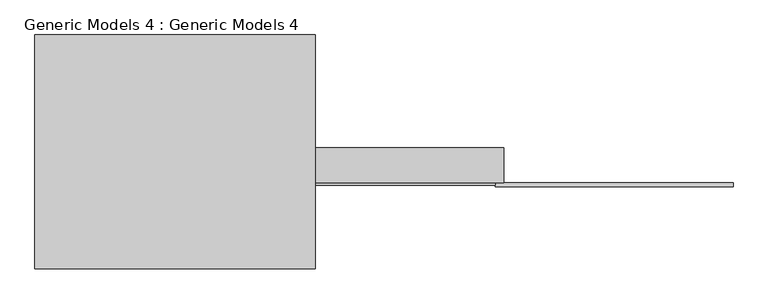
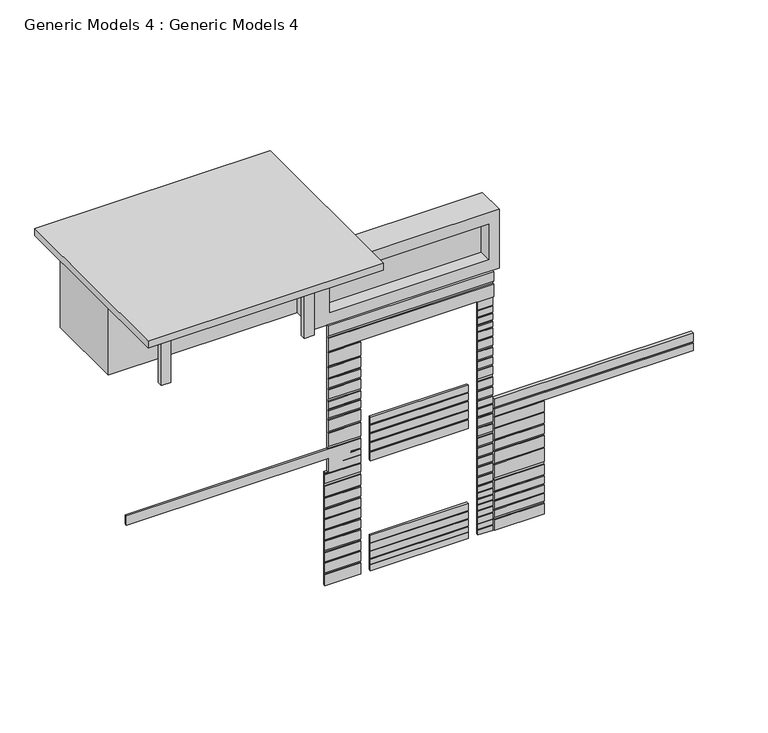
"""IFC4 building model written with IfcOpenShell, lengths in millimetres: proxy geometry, Generic Models 4 : Generic Models 4."""

from ifc_helpers import new_model, si_unit, frame, origin, place, context, project, spatial, polyline, outline, extrude, faceted_brep, source, transform, mapped, element, save


def generic_models_4_generic_models_4_71b53b29(model_context):
    return source(origin(), model_context, "Body", "SolidModel", [
        extrude(outline(polyline([(-14860.146149, 871.6720769), (-14860.146149, 0.0), (-14910.946149, 0.0), (-14910.946149, 143.2262452), (-14885.546149, 143.2262452), (-14885.546149, 160.2144956), (-14910.946149, 160.2144956), (-14910.946149, 282.4741118), (-14885.546149, 282.4741118), (-14885.546149, 303.6396643), (-14910.946149, 303.6396643), (-14910.946149, 472.2042083), (-14885.546149, 472.2042083), (-14885.546149, 489.55907), (-14910.946149, 489.55907), (-14910.946149, 670.6560858), (-14885.546149, 670.6560858), (-14885.546149, 693.359854), (-14910.946149, 693.359854), (-14910.946149, 871.6720769), (-14860.146149, 871.6720769)])), frame((-13085.9127168, 0.0, 0.0), z_axis=(1.0, 0.0, 0.0), x_axis=(0.0, 1.0, 0.0)), (0.0, 0.0, 1.0), 2286.0),
        extrude(outline(polyline([(-14860.146149, 3795.2224075), (-14860.146149, 2722.517897), (-14910.946149, 2722.517897), (-14910.946149, 2926.2507447), (-14885.546149, 2926.2507447), (-14885.546149, 2967.5143081), (-14910.946149, 2967.5143081), (-14910.946149, 3162.0425355), (-14885.546149, 3162.0425355), (-14885.546149, 3197.4113041), (-14910.946149, 3197.4113041), (-14910.946149, 3386.0447367), (-14885.546149, 3386.0447367), (-14885.546149, 3424.3609027), (-14910.946149, 3424.3609027), (-14910.946149, 3598.2573484), (-14885.546149, 3598.2573484), (-14885.546149, 3630.9088336), (-14910.946149, 3630.9088336), (-14910.946149, 3795.2224075), (-14860.146149, 3795.2224075)])), frame((-13085.9127168, 0.0, 0.0), z_axis=(1.0, 0.0, 0.0), x_axis=(0.0, 1.0, 0.0)), (0.0, 0.0, 1.0), 2286.0),
        faceted_brep([(-10203.7104375, -14936.346149, 0.0), (-9027.8261094, -14936.346149, 0.0), (-9027.8261094, -14936.346149, 264.8835225), (-10203.7104375, -14936.346149, 264.8835225), (-5541.6761094, -14936.346149, 3259.8014539), (-10203.7104375, -14936.346149, 3259.8014539), (-10203.7104375, -14936.346149, 3048.0), (-5541.6761094, -14936.346149, 3048.0), (-10203.7104375, -14936.346149, 2798.9145678), (-10203.7104375, -14936.346149, 2536.7442955), (-9027.8261094, -14936.346149, 2536.7442955), (-9027.8261094, -14936.346149, 2798.9145678), (-10203.7104375, -14936.346149, 2510.3531457), (-10203.7104375, -14936.346149, 2253.5396211), (-9027.8261094, -14936.346149, 2253.5396211), (-9027.8261094, -14936.346149, 2510.3531457), (-10203.7104375, -14936.346149, 2219.6445512), (-10203.7104375, -14936.346149, 1992.5475827), (-9027.8261094, -14936.346149, 1992.5475827), (-9027.8261094, -14936.346149, 2219.6445512), (-10203.7104375, -14936.346149, 1945.0944848), (-10203.7104375, -14936.346149, 1662.3980138), (-9027.8261094, -14936.346149, 1662.3980138), (-9027.8261094, -14936.346149, 1945.0944848), (-10203.7104375, -14936.346149, 1629.900727), (-10203.7104375, -14936.346149, 1299.305551), (-9027.8261094, -14936.346149, 1299.305551), (-9027.8261094, -14936.346149, 1629.900727), (-10203.7104375, -14936.346149, 1226.3227773), (-10203.7104375, -14936.346149, 979.6915986), (-9027.8261094, -14936.346149, 979.6915986), (-9027.8261094, -14936.346149, 1226.3227773), (-10203.7104375, -14936.346149, 946.2617606), (-10203.7104375, -14936.346149, 759.0546678), (-9027.8261094, -14936.346149, 759.0546678), (-9027.8261094, -14936.346149, 946.2617606), (-10203.7104375, -14936.346149, 502.759243), (-10203.7104375, -14936.346149, 321.8090911), (-9027.8261094, -14936.346149, 321.8090911), (-9027.8261094, -14936.346149, 502.759243), (-10203.7104375, -14936.346149, 723.3961739), (-10203.7104375, -14936.346149, 537.8317429), (-9027.8261094, -14936.346149, 537.8317429), (-9027.8261094, -14936.346149, 723.3961739), (-10203.7104375, -14936.346149, 2829.1963889), (-5541.6761094, -14936.346149, 2829.1963889), (-5541.6761094, -14936.346149, 3017.3784928), (-10203.7104375, -14936.346149, 3017.3784928), (-9027.8261094, -14860.146149, 0.0), (-10203.7104375, -14860.146149, 0.0), (-10203.7104375, -14860.146149, 3259.8014539), (-5541.6761094, -14860.146149, 3259.8014539), (-5541.6761094, -14860.146149, 2829.1963889), (-9027.8261094, -14860.146149, 2829.1963889), (-10203.7104375, -14910.946149, 264.8835225), (-10203.7104375, -14910.946149, 321.8090911), (-10203.7104375, -14910.946149, 502.759243), (-10203.7104375, -14910.946149, 537.8317429), (-10203.7104375, -14910.946149, 723.3961739), (-10203.7104375, -14910.946149, 759.0546678), (-10203.7104375, -14910.946149, 946.2617606), (-10203.7104375, -14910.946149, 979.6915986), (-10203.7104375, -14910.946149, 1226.3227773), (-10203.7104375, -14910.946149, 1299.305551), (-10203.7104375, -14910.946149, 1629.900727), (-10203.7104375, -14910.946149, 1662.3980138), (-10203.7104375, -14910.946149, 1945.0944848), (-10203.7104375, -14910.946149, 1992.5475827), (-10203.7104375, -14910.946149, 2219.6445512), (-10203.7104375, -14910.946149, 2253.5396211), (-10203.7104375, -14910.946149, 2510.3531457), (-10203.7104375, -14910.946149, 2536.7442955), (-10203.7104375, -14910.946149, 2798.9145678), (-10203.7104375, -14910.946149, 2829.1963889), (-10203.7104375, -14910.946149, 3017.3784928), (-10203.7104375, -14910.946149, 3048.0), (-9027.8261094, -14910.946149, 2829.1963889), (-9027.8261094, -14910.946149, 2798.9145678), (-9027.8261094, -14910.946149, 2536.7442955), (-9027.8261094, -14910.946149, 2510.3531457), (-9027.8261094, -14910.946149, 2253.5396211), (-9027.8261094, -14910.946149, 2219.6445512), (-9027.8261094, -14910.946149, 1992.5475827), (-9027.8261094, -14910.946149, 1945.0944848), (-9027.8261094, -14910.946149, 1662.3980138), (-9027.8261094, -14910.946149, 1629.900727), (-9027.8261094, -14910.946149, 1299.305551), (-9027.8261094, -14910.946149, 1226.3227773), (-9027.8261094, -14910.946149, 979.6915986), (-9027.8261094, -14910.946149, 946.2617606), (-9027.8261094, -14910.946149, 759.0546678), (-9027.8261094, -14910.946149, 723.3961739), (-9027.8261094, -14910.946149, 537.8317429), (-9027.8261094, -14910.946149, 502.759243), (-9027.8261094, -14910.946149, 321.8090911), (-9027.8261094, -14910.946149, 264.8835225), (-5541.6761094, -14910.946149, 3048.0), (-5541.6761094, -14910.946149, 3017.3784928)], [[[0, 1, 2, 3]], [[4, 5, 6, 7]], [[8, 9, 10, 11]], [[12, 13, 14, 15]], [[16, 17, 18, 19]], [[20, 21, 22, 23]], [[24, 25, 26, 27]], [[28, 29, 30, 31]], [[32, 33, 34, 35]], [[36, 37, 38, 39]], [[40, 41, 42, 43]], [[44, 45, 46, 47]], [[48, 49, 50, 51, 52, 53]], [[50, 5, 4, 51]], [[50, 49, 0, 3, 54, 55, 37, 36, 56, 57, 41, 40, 58, 59, 33, 32, 60, 61, 29, 28, 62, 63, 25, 24, 64, 65, 21, 20, 66, 67, 17, 16, 68, 69, 13, 12, 70, 71, 9, 8, 72, 73, 44, 47, 74, 75, 6, 5]], [[1, 0, 49, 48]], [[1, 48, 53, 76, 77, 11, 10, 78, 79, 15, 14, 80, 81, 19, 18, 82, 83, 23, 22, 84, 85, 27, 26, 86, 87, 31, 30, 88, 89, 35, 34, 90, 91, 43, 42, 92, 93, 39, 38, 94, 95, 2]], [[44, 73, 76, 53, 52, 45]], [[52, 51, 4, 7, 96, 97, 46, 45]], [[72, 77, 76, 73]], [[70, 79, 78, 71]], [[68, 81, 80, 69]], [[66, 83, 82, 67]], [[64, 85, 84, 65]], [[88, 61, 60, 89]], [[90, 59, 58, 91]], [[92, 57, 56, 93]], [[96, 75, 74, 97]], [[62, 87, 86, 63]], [[54, 95, 94, 55]], [[77, 72, 8, 11]], [[71, 78, 10, 9]], [[79, 70, 12, 15]], [[69, 80, 14, 13]], [[81, 68, 16, 19]], [[67, 82, 18, 17]], [[83, 66, 20, 23]], [[65, 84, 22, 21]], [[85, 64, 24, 27]], [[63, 86, 26, 25]], [[87, 62, 28, 31]], [[55, 94, 38, 37]], [[95, 54, 3, 2]], [[89, 60, 32, 35]], [[61, 88, 30, 29]], [[91, 58, 40, 43]], [[59, 90, 34, 33]], [[93, 56, 36, 39]], [[57, 92, 42, 41]], [[97, 74, 47, 46]], [[75, 96, 7, 6]]]),
        faceted_brep([(-10571.3127168, -14860.146149, 0.0), (-10571.3127168, -14910.946149, 0.0), (-10571.3127168, -14910.946149, 118.2725127), (-10571.3127168, -14885.546149, 118.2725127), (-10571.3127168, -14885.546149, 145.235457), (-10571.3127168, -14910.946149, 145.235457), (-10571.3127168, -14910.946149, 264.8835225), (-10571.3127168, -14885.546149, 264.8835225), (-10571.3127168, -14885.546149, 281.7353627), (-10571.3127168, -14910.946149, 281.7353627), (-10571.3127168, -14910.946149, 424.9760045), (-10571.3127168, -14885.546149, 424.9760045), (-10571.3127168, -14885.546149, 451.9389488), (-10571.3127168, -14910.946149, 451.9389488), (-10571.3127168, -14910.946149, 583.3833024), (-10571.3127168, -14885.546149, 583.3833024), (-10571.3127168, -14885.546149, 608.6610627), (-10571.3127168, -14910.946149, 608.6610627), (-10571.3127168, -14910.946149, 731.6794962), (-10571.3127168, -14885.546149, 731.6794962), (-10571.3127168, -14885.546149, 758.6424406), (-10571.3127168, -14910.946149, 758.6424406), (-10571.3127168, -14910.946149, 871.6720769), (-10571.3127168, -14885.546149, 871.6720769), (-10571.3127168, -14885.546149, 903.5682663), (-10571.3127168, -14910.946149, 903.5682663), (-10571.3127168, -14910.946149, 1031.1366967), (-10571.3127168, -14885.546149, 1031.1366967), (-10571.3127168, -14885.546149, 1058.2681594), (-10571.3127168, -14910.946149, 1058.2681594), (-10571.3127168, -14910.946149, 1195.8634347), (-10571.3127168, -14885.546149, 1195.8634347), (-10571.3127168, -14885.546149, 1226.3227773), (-10571.3127168, -14910.946149, 1226.3227773), (-10571.3127168, -14910.946149, 1416.1351688), (-10571.3127168, -14885.546149, 1416.1351688), (-10571.3127168, -14885.546149, 1470.3672807), (-10571.3127168, -14910.946149, 1470.3672807), (-10571.3127168, -14910.946149, 1663.5691793), (-10571.3127168, -14885.546149, 1663.5691793), (-10571.3127168, -14885.546149, 1711.0222772), (-10571.3127168, -14910.946149, 1711.0222772), (-10571.3127168, -14910.946149, 1887.2766408), (-10571.3127168, -14885.546149, 1887.2766408), (-10571.3127168, -14885.546149, 1938.1192457), (-10571.3127168, -14910.946149, 1938.1192457), (-10571.3127168, -14910.946149, 2141.4896652), (-10571.3127168, -14885.546149, 2141.4896652), (-10571.3127168, -14885.546149, 2202.500791), (-10571.3127168, -14910.946149, 2202.500791), (-10571.3127168, -14910.946149, 2395.7026896), (-10571.3127168, -14885.546149, 2395.7026896), (-10571.3127168, -14885.546149, 2460.1033225), (-10571.3127168, -14910.946149, 2460.1033225), (-10571.3127168, -14910.946149, 2636.3576861), (-10571.3127168, -14885.546149, 2636.3576861), (-10571.3127168, -14885.546149, 2697.3688119), (-10571.3127168, -14910.946149, 2697.3688119), (-10571.3127168, -14910.946149, 2892.8888996), (-10571.3127168, -14885.546149, 2892.8888996), (-10571.3127168, -14885.546149, 2944.8028224), (-10571.3127168, -14910.946149, 2944.8028224), (-10571.3127168, -14910.946149, 3110.888665), (-10571.3127168, -14885.546149, 3110.888665), (-10571.3127168, -14885.546149, 3154.9522559), (-10571.3127168, -14910.946149, 3154.9522559), (-10571.3127168, -14910.946149, 3307.4800705), (-10571.3127168, -14885.546149, 3307.4800705), (-10571.3127168, -14885.546149, 3358.3226754), (-10571.3127168, -14910.946149, 3358.3226754), (-10571.3127168, -14910.946149, 3544.74556), (-10571.3127168, -14885.546149, 3544.74556), (-10571.3127168, -14885.546149, 3595.5881649), (-10571.3127168, -14910.946149, 3595.5881649), (-10571.3127168, -14910.946149, 3795.2224075), (-10571.3127168, -14885.546149, 3795.2224075), (-10571.3127168, -14885.546149, 3866.7487242), (-10571.3127168, -14910.946149, 3866.7487242), (-10571.3127168, -14910.946149, 4059.9506228), (-10571.3127168, -14885.546149, 4059.9506228), (-10571.3127168, -14885.546149, 4114.1827347), (-10571.3127168, -14910.946149, 4114.1827347), (-10571.3127168, -14910.946149, 4285.3602063), (-10571.3127168, -14885.546149, 4285.3602063), (-10571.3127168, -14885.546149, 4336.2028112), (-10571.3127168, -14910.946149, 4336.2028112), (-10571.3127168, -14910.946149, 4529.4047097), (-10571.3127168, -14885.546149, 4529.4047097), (-10571.3127168, -14885.546149, 4580.2473146), (-10571.3127168, -14910.946149, 4580.2473146), (-10571.3127168, -14910.946149, 4780.2282272), (-10571.3127168, -14885.546149, 4780.2282272), (-10571.3127168, -14885.546149, 4824.2918181), (-10571.3127168, -14910.946149, 4824.2918181), (-10571.3127168, -14910.946149, 5011.9601219), (-10571.3127168, -14885.546149, 5011.9601219), (-10571.3127168, -14885.546149, 5043.161304), (-10571.3127168, -14910.946149, 5043.161304), (-10571.3127168, -14910.946149, 5172.4233443), (-10571.3127168, -14885.546149, 5172.4233443), (-10571.3127168, -14885.546149, 5219.2251175), (-10571.3127168, -14910.946149, 5219.2251175), (-10571.3127168, -14910.946149, 5361.859093), (-10571.3127168, -14885.546149, 5361.859093), (-10571.3127168, -14885.546149, 5397.5175869), (-10571.3127168, -14910.946149, 5397.5175869), (-10571.3127168, -14910.946149, 5544.6088742), (-10571.3127168, -14885.546149, 5544.6088742), (-10571.3127168, -14885.546149, 5574.6202549), (-10571.3127168, -14910.946149, 5574.6202549), (-10571.3127168, -14910.946149, 5768.9220842), (-10571.3127168, -14885.546149, 5768.9220842), (-10571.3127168, -14885.546149, 5777.8202549), (-10571.3127168, -14910.946149, 5777.8202549), (-10571.3127168, -14910.946149, 5785.7777992), (-10571.3127168, -14860.146149, 5785.7777992), (-10219.8600301, -14910.946149, 0.0), (-10219.8600301, -14860.146149, 0.0), (-10219.8600301, -14860.146149, 5785.7777992), (-10219.8600301, -14910.946149, 5785.7777992), (-10219.8600301, -14910.946149, 5777.8202549), (-10219.8600301, -14885.546149, 5777.8202549), (-10219.8600301, -14885.546149, 5768.9220842), (-10219.8600301, -14910.946149, 5768.9220842), (-10219.8600301, -14910.946149, 5574.6202549), (-10219.8600301, -14885.546149, 5574.6202549), (-10219.8600301, -14885.546149, 5544.6088742), (-10219.8600301, -14910.946149, 5544.6088742), (-10219.8600301, -14910.946149, 5397.5175869), (-10219.8600301, -14885.546149, 5397.5175869), (-10219.8600301, -14885.546149, 5361.859093), (-10219.8600301, -14910.946149, 5361.859093), (-10219.8600301, -14910.946149, 5219.2251175), (-10219.8600301, -14885.546149, 5219.2251175), (-10219.8600301, -14885.546149, 5172.4233443), (-10219.8600301, -14910.946149, 5172.4233443), (-10219.8600301, -14910.946149, 5043.161304), (-10219.8600301, -14885.546149, 5043.161304), (-10219.8600301, -14885.546149, 5011.9601219), (-10219.8600301, -14910.946149, 5011.9601219), (-10219.8600301, -14910.946149, 4824.2918181), (-10219.8600301, -14885.546149, 4824.2918181), (-10219.8600301, -14885.546149, 4780.2282272), (-10219.8600301, -14910.946149, 4780.2282272), (-10219.8600301, -14910.946149, 4580.2473146), (-10219.8600301, -14885.546149, 4580.2473146), (-10219.8600301, -14885.546149, 4529.4047097), (-10219.8600301, -14910.946149, 4529.4047097), (-10219.8600301, -14910.946149, 4336.2028112), (-10219.8600301, -14885.546149, 4336.2028112), (-10219.8600301, -14885.546149, 4285.3602063), (-10219.8600301, -14910.946149, 4285.3602063), (-10219.8600301, -14910.946149, 4114.1827347), (-10219.8600301, -14885.546149, 4114.1827347), (-10219.8600301, -14885.546149, 4059.9506228), (-10219.8600301, -14910.946149, 4059.9506228), (-10219.8600301, -14910.946149, 3866.7487242), (-10219.8600301, -14885.546149, 3866.7487242), (-10219.8600301, -14885.546149, 3795.2224075), (-10219.8600301, -14910.946149, 3795.2224075), (-10219.8600301, -14910.946149, 3595.5881649), (-10219.8600301, -14885.546149, 3595.5881649), (-10219.8600301, -14885.546149, 3544.74556), (-10219.8600301, -14910.946149, 3544.74556), (-10219.8600301, -14910.946149, 3358.3226754), (-10219.8600301, -14885.546149, 3358.3226754), (-10219.8600301, -14885.546149, 3307.4800705), (-10219.8600301, -14910.946149, 3307.4800705), (-10219.8600301, -14910.946149, 3154.9522559), (-10219.8600301, -14885.546149, 3154.9522559), (-10219.8600301, -14885.546149, 3110.888665), (-10219.8600301, -14910.946149, 3110.888665), (-10219.8600301, -14910.946149, 2944.8028224), (-10219.8600301, -14885.546149, 2944.8028224), (-10219.8600301, -14885.546149, 2892.8888996), (-10219.8600301, -14910.946149, 2892.8888996), (-10219.8600301, -14910.946149, 2697.3688119), (-10219.8600301, -14885.546149, 2697.3688119), (-10219.8600301, -14885.546149, 2636.3576861), (-10219.8600301, -14910.946149, 2636.3576861), (-10219.8600301, -14910.946149, 2460.1033225), (-10219.8600301, -14885.546149, 2460.1033225), (-10219.8600301, -14885.546149, 2395.7026896), (-10219.8600301, -14910.946149, 2395.7026896), (-10219.8600301, -14910.946149, 2202.500791), (-10219.8600301, -14885.546149, 2202.500791), (-10219.8600301, -14885.546149, 2141.4896652), (-10219.8600301, -14910.946149, 2141.4896652), (-10219.8600301, -14910.946149, 1938.1192457), (-10219.8600301, -14885.546149, 1938.1192457), (-10219.8600301, -14885.546149, 1887.2766408), (-10219.8600301, -14910.946149, 1887.2766408), (-10219.8600301, -14910.946149, 1711.0222772), (-10219.8600301, -14885.546149, 1711.0222772), (-10219.8600301, -14885.546149, 1663.5691793), (-10219.8600301, -14910.946149, 1663.5691793), (-10219.8600301, -14910.946149, 1470.3672807), (-10219.8600301, -14885.546149, 1470.3672807), (-10219.8600301, -14885.546149, 1416.1351688), (-10219.8600301, -14910.946149, 1416.1351688), (-10219.8600301, -14910.946149, 1226.3227773), (-10219.8600301, -14885.546149, 1226.3227773), (-10219.8600301, -14885.546149, 1195.8634347), (-10219.8600301, -14910.946149, 1195.8634347), (-10219.8600301, -14910.946149, 1058.2681594), (-10219.8600301, -14885.546149, 1058.2681594), (-10219.8600301, -14885.546149, 1031.1366967), (-10219.8600301, -14910.946149, 1031.1366967), (-10219.8600301, -14910.946149, 903.5682663), (-10219.8600301, -14885.546149, 903.5682663), (-10219.8600301, -14885.546149, 871.6720769), (-10219.8600301, -14910.946149, 871.6720769), (-10219.8600301, -14910.946149, 758.6424406), (-10219.8600301, -14885.546149, 758.6424406), (-10219.8600301, -14885.546149, 731.6794962), (-10219.8600301, -14910.946149, 731.6794962), (-10219.8600301, -14910.946149, 608.6610627), (-10219.8600301, -14885.546149, 608.6610627), (-10219.8600301, -14885.546149, 583.3833024), (-10219.8600301, -14910.946149, 583.3833024), (-10219.8600301, -14910.946149, 451.9389488), (-10219.8600301, -14885.546149, 451.9389488), (-10219.8600301, -14885.546149, 424.9760045), (-10219.8600301, -14910.946149, 424.9760045), (-10219.8600301, -14910.946149, 281.7353627), (-10219.8600301, -14885.546149, 281.7353627), (-10219.8600301, -14885.546149, 264.8835225), (-10219.8600301, -14910.946149, 264.8835225), (-10219.8600301, -14910.946149, 145.235457), (-10219.8600301, -14885.546149, 145.235457), (-10219.8600301, -14885.546149, 118.2725127), (-10219.8600301, -14910.946149, 118.2725127), (-14076.5127168, -14910.946149, 6400.8), (-10203.7104375, -14910.946149, 6400.8), (-10203.7104375, -14860.146149, 6400.8), (-14076.5127168, -14860.146149, 6400.8), (-10203.7104375, -14860.146149, 5785.7777992), (-10203.7104375, -14910.946149, 5785.7777992), (-13314.5127168, -14910.946149, 5785.7777992), (-13314.5127168, -14860.146149, 5785.7777992), (-10203.7104375, -14910.946149, 6157.8924204), (-10203.7104375, -14885.546149, 6157.8924204), (-10203.7104375, -14885.546149, 6093.2888996), (-10203.7104375, -14910.946149, 6093.2888996), (-14076.5127168, -14910.946149, 6157.8924204), (-14076.5127168, -14910.946149, 2794.612741), (-14152.2761094, -14910.946149, 2794.612741), (-14152.2761094, -14910.946149, 2764.0290782), (-13314.5127168, -14910.946149, 2764.0290782), (-13314.5127168, -14910.946149, 2941.3397448), (-13733.3783685, -14910.946149, 2941.3397448), (-13733.3783685, -14910.946149, 2958.9242737), (-13314.5127168, -14910.946149, 2958.9242737), (-13314.5127168, -14910.946149, 3093.7389953), (-13549.4767283, -14910.946149, 3093.7389953), (-13549.4767283, -14910.946149, 3124.2), (-13314.5127168, -14910.946149, 3124.2), (-13314.5127168, -14910.946149, 3352.8), (-18800.4761094, -14910.946149, 3352.8), (-18800.4761094, -14910.946149, 3124.2), (-14076.5127168, -14910.946149, 3124.2), (-14152.2761094, -14910.946149, 0.0), (-13314.5127168, -14910.946149, 0.0), (-13314.5127168, -14910.946149, 271.0579363), (-14152.2761094, -14910.946149, 271.0579363), (-14076.5127168, -14910.946149, 6093.2888996), (-14076.5127168, -14910.946149, 5777.8202549), (-13314.5127168, -14910.946149, 5777.8202549), (-13314.5127168, -14910.946149, 5413.0434819), (-13314.5127168, -14910.946149, 5738.8584125), (-14076.5127168, -14910.946149, 5738.8584125), (-14076.5127168, -14910.946149, 5413.0434819), (-13314.5127168, -14910.946149, 5123.3890782), (-13314.5127168, -14910.946149, 5370.3472182), (-14076.5127168, -14910.946149, 5370.3472182), (-14076.5127168, -14910.946149, 5123.3890782), (-13314.5127168, -14910.946149, 4876.8), (-13314.5127168, -14910.946149, 5080.0), (-14076.5127168, -14910.946149, 5080.0), (-14076.5127168, -14910.946149, 4876.8), (-13314.5127168, -14910.946149, 4597.7063705), (-13314.5127168, -14910.946149, 4824.2918181), (-14076.5127168, -14910.946149, 4824.2918181), (-14076.5127168, -14910.946149, 4597.7063705), (-13314.5127168, -14910.946149, 4356.692968), (-13314.5127168, -14910.946149, 4529.4047097), (-14076.5127168, -14910.946149, 4529.4047097), (-14076.5127168, -14910.946149, 4356.692968), (-13314.5127168, -14910.946149, 4123.7486803), (-13314.5127168, -14910.946149, 4307.942964), (-14076.5127168, -14910.946149, 4307.942964), (-14076.5127168, -14910.946149, 4123.7486803), (-13314.5127168, -14910.946149, 3795.2224075), (-13314.5127168, -14910.946149, 4073.0755508), (-14076.5127168, -14910.946149, 4073.0755508), (-14076.5127168, -14910.946149, 3795.2224075), (-13314.5127168, -14910.946149, 3418.2227999), (-13314.5127168, -14910.946149, 3745.6491753), (-14076.5127168, -14910.946149, 3745.6491753), (-14076.5127168, -14910.946149, 3418.2227999), (-13314.5127168, -14910.946149, 2536.7442955), (-13314.5127168, -14910.946149, 2742.0484171), (-14152.2761094, -14910.946149, 2742.0484171), (-14152.2761094, -14910.946149, 2536.7442955), (-13314.5127168, -14910.946149, 2202.500791), (-13314.5127168, -14910.946149, 2460.1033225), (-14152.2761094, -14910.946149, 2460.1033225), (-14152.2761094, -14910.946149, 2202.500791), (-13314.5127168, -14910.946149, 1928.5268555), (-13314.5127168, -14910.946149, 2159.013331), (-14152.2761094, -14910.946149, 2159.013331), (-14152.2761094, -14910.946149, 1928.5268555), (-13314.5127168, -14910.946149, 1664.1453101), (-13314.5127168, -14910.946149, 1881.0737576), (-14152.2761094, -14910.946149, 1881.0737576), (-14152.2761094, -14910.946149, 1664.1453101), (-13314.5127168, -14910.946149, 1397.3063705), (-13314.5127168, -14910.946149, 1630.2502402), (-14152.2761094, -14910.946149, 1630.2502402), (-14152.2761094, -14910.946149, 1397.3063705), (-13314.5127168, -14910.946149, 1138.7717263), (-13314.5127168, -14910.946149, 1355.7001738), (-14152.2761094, -14910.946149, 1355.7001738), (-14152.2761094, -14910.946149, 1138.7717263), (-13314.5127168, -14910.946149, 871.6720769), (-13314.5127168, -14910.946149, 1094.7081354), (-14152.2761094, -14910.946149, 1094.7081354), (-14152.2761094, -14910.946149, 871.6720769), (-13314.5127168, -14910.946149, 589.6715936), (-13314.5127168, -14910.946149, 820.1580691), (-14152.2761094, -14910.946149, 820.1580691), (-14152.2761094, -14910.946149, 589.6715936), (-13314.5127168, -14910.946149, 325.2900482), (-13314.5127168, -14910.946149, 552.3870167), (-14152.2761094, -14910.946149, 552.3870167), (-14152.2761094, -14910.946149, 325.2900482), (-13314.5127168, -14860.146149, 0.0), (-14152.2761094, -14860.146149, 0.0), (-14152.2761094, -14860.146149, 2794.612741), (-14076.5127168, -14860.146149, 2794.612741), (-14076.5127168, -14860.146149, 3124.2), (-18800.4761094, -14860.146149, 3124.2), (-18800.4761094, -14860.146149, 3352.8), (-14076.5127168, -14860.146149, 3352.8), (-14076.5127168, -14885.546149, 3352.8), (-14076.5127168, -14885.546149, 3418.2227999), (-14076.5127168, -14885.546149, 3745.6491753), (-14076.5127168, -14885.546149, 3795.2224075), (-14076.5127168, -14885.546149, 4073.0755508), (-14076.5127168, -14885.546149, 4123.7486803), (-14076.5127168, -14885.546149, 4307.942964), (-14076.5127168, -14885.546149, 4356.692968), (-14076.5127168, -14885.546149, 4529.4047097), (-14076.5127168, -14885.546149, 4597.7063705), (-14076.5127168, -14885.546149, 4824.2918181), (-14076.5127168, -14885.546149, 4876.8), (-14076.5127168, -14885.546149, 5080.0), (-14076.5127168, -14885.546149, 5123.3890782), (-14076.5127168, -14885.546149, 5370.3472182), (-14076.5127168, -14885.546149, 5413.0434819), (-14076.5127168, -14885.546149, 5738.8584125), (-14076.5127168, -14885.546149, 5777.8202549), (-14076.5127168, -14885.546149, 6093.2888996), (-14076.5127168, -14885.546149, 6157.8924204), (-13314.5127168, -14885.546149, 5777.8202549), (-13314.5127168, -14885.546149, 5738.8584125), (-13314.5127168, -14885.546149, 5413.0434819), (-13314.5127168, -14885.546149, 5370.3472182), (-13314.5127168, -14885.546149, 5123.3890782), (-13314.5127168, -14885.546149, 5080.0), (-13314.5127168, -14885.546149, 4876.8), (-13314.5127168, -14885.546149, 4824.2918181), (-13314.5127168, -14885.546149, 4597.7063705), (-13314.5127168, -14885.546149, 4529.4047097), (-13314.5127168, -14885.546149, 4356.692968), (-13314.5127168, -14885.546149, 4307.942964), (-13314.5127168, -14885.546149, 4123.7486803), (-13314.5127168, -14885.546149, 4073.0755508), (-13314.5127168, -14885.546149, 3795.2224075), (-13314.5127168, -14885.546149, 3745.6491753), (-13314.5127168, -14885.546149, 3418.2227999), (-13314.5127168, -14885.546149, 3352.8), (-13314.5127168, -14885.546149, 3124.2), (-13314.5127168, -14885.546149, 3093.7389953), (-13314.5127168, -14885.546149, 2958.9242737), (-13314.5127168, -14885.546149, 2941.3397448), (-13314.5127168, -14885.546149, 2764.0290782), (-13314.5127168, -14885.546149, 2742.0484171), (-13314.5127168, -14885.546149, 2536.7442955), (-13314.5127168, -14885.546149, 2460.1033225), (-13314.5127168, -14885.546149, 2202.500791), (-13314.5127168, -14885.546149, 2159.013331), (-13314.5127168, -14885.546149, 1928.5268555), (-13314.5127168, -14885.546149, 1881.0737576), (-13314.5127168, -14885.546149, 1664.1453101), (-13314.5127168, -14885.546149, 1630.2502402), (-13314.5127168, -14885.546149, 1397.3063705), (-13314.5127168, -14885.546149, 1355.7001738), (-13314.5127168, -14885.546149, 1138.7717263), (-13314.5127168, -14885.546149, 1094.7081354), (-13314.5127168, -14885.546149, 871.6720769), (-13314.5127168, -14885.546149, 820.1580691), (-13314.5127168, -14885.546149, 589.6715936), (-13314.5127168, -14885.546149, 552.3870167), (-13314.5127168, -14885.546149, 325.2900482), (-13314.5127168, -14885.546149, 271.0579363), (-14152.2761094, -14885.546149, 271.0579363), (-14152.2761094, -14885.546149, 325.2900482), (-14152.2761094, -14885.546149, 552.3870167), (-14152.2761094, -14885.546149, 589.6715936), (-14152.2761094, -14885.546149, 820.1580691), (-14152.2761094, -14885.546149, 871.6720769), (-14152.2761094, -14885.546149, 1094.7081354), (-14152.2761094, -14885.546149, 1138.7717263), (-14152.2761094, -14885.546149, 1355.7001738), (-14152.2761094, -14885.546149, 1397.3063705), (-14152.2761094, -14885.546149, 1630.2502402), (-14152.2761094, -14885.546149, 1664.1453101), (-14152.2761094, -14885.546149, 1881.0737576), (-14152.2761094, -14885.546149, 1928.5268555), (-14152.2761094, -14885.546149, 2159.013331), (-14152.2761094, -14885.546149, 2202.500791), (-14152.2761094, -14885.546149, 2460.1033225), (-14152.2761094, -14885.546149, 2536.7442955), (-14152.2761094, -14885.546149, 2742.0484171), (-14152.2761094, -14885.546149, 2764.0290782), (-13549.4767283, -14885.546149, 3124.2), (-13549.4767283, -14885.546149, 3093.7389953), (-13733.3783685, -14885.546149, 2958.9242737), (-13733.3783685, -14885.546149, 2941.3397448)], [[[0, 1, 2, 3, 4, 5, 6, 7, 8, 9, 10, 11, 12, 13, 14, 15, 16, 17, 18, 19, 20, 21, 22, 23, 24, 25, 26, 27, 28, 29, 30, 31, 32, 33, 34, 35, 36, 37, 38, 39, 40, 41, 42, 43, 44, 45, 46, 47, 48, 49, 50, 51, 52, 53, 54, 55, 56, 57, 58, 59, 60, 61, 62, 63, 64, 65, 66, 67, 68, 69, 70, 71, 72, 73, 74, 75, 76, 77, 78, 79, 80, 81, 82, 83, 84, 85, 86, 87, 88, 89, 90, 91, 92, 93, 94, 95, 96, 97, 98, 99, 100, 101, 102, 103, 104, 105, 106, 107, 108, 109, 110, 111, 112, 113, 114, 115]], [[116, 1, 0, 117]], [[116, 117, 118, 119, 120, 121, 122, 123, 124, 125, 126, 127, 128, 129, 130, 131, 132, 133, 134, 135, 136, 137, 138, 139, 140, 141, 142, 143, 144, 145, 146, 147, 148, 149, 150, 151, 152, 153, 154, 155, 156, 157, 158, 159, 160, 161, 162, 163, 164, 165, 166, 167, 168, 169, 170, 171, 172, 173, 174, 175, 176, 177, 178, 179, 180, 181, 182, 183, 184, 185, 186, 187, 188, 189, 190, 191, 192, 193, 194, 195, 196, 197, 198, 199, 200, 201, 202, 203, 204, 205, 206, 207, 208, 209, 210, 211, 212, 213, 214, 215, 216, 217, 218, 219, 220, 221, 222, 223, 224, 225, 226, 227, 228, 229, 230, 231]], [[232, 233, 234, 235]], [[236, 237, 119, 118]], [[238, 239, 115, 114]], [[236, 234, 233, 240, 241, 242, 243, 237]], [[1, 116, 231, 2]], [[233, 232, 244, 240]], [[245, 246, 247, 248, 249, 250, 251, 252, 253, 254, 255, 256, 257, 258, 259, 260]], [[261, 262, 263, 264]], [[238, 114, 113, 120, 119, 237, 243, 265, 266, 267]], [[268, 269, 270, 271]], [[272, 273, 274, 275]], [[276, 277, 278, 279]], [[280, 281, 282, 283]], [[284, 285, 286, 287]], [[288, 289, 290, 291]], [[292, 293, 294, 295]], [[296, 297, 298, 299]], [[300, 301, 302, 303]], [[304, 305, 306, 307]], [[308, 309, 310, 311]], [[312, 313, 314, 315]], [[316, 317, 318, 319]], [[320, 321, 322, 323]], [[324, 325, 326, 327]], [[328, 329, 330, 331]], [[332, 333, 334, 335]], [[110, 109, 124, 123]], [[106, 105, 128, 127]], [[102, 101, 132, 131]], [[98, 97, 136, 135]], [[94, 93, 140, 139]], [[90, 89, 144, 143]], [[86, 85, 148, 147]], [[82, 81, 152, 151]], [[78, 77, 156, 155]], [[74, 73, 160, 159]], [[70, 69, 164, 163]], [[66, 65, 168, 167]], [[62, 61, 172, 171]], [[58, 57, 176, 175]], [[54, 53, 180, 179]], [[50, 49, 184, 183]], [[46, 45, 188, 187]], [[42, 41, 192, 191]], [[38, 37, 196, 195]], [[34, 33, 200, 199]], [[30, 29, 204, 203]], [[26, 25, 208, 207]], [[22, 21, 212, 211]], [[18, 17, 216, 215]], [[14, 13, 220, 219]], [[10, 9, 224, 223]], [[6, 5, 228, 227]], [[239, 336, 337, 338, 339, 340, 341, 342, 343, 235, 234, 236, 118, 117, 0, 115]], [[232, 235, 343, 344, 345, 299, 298, 346, 347, 295, 294, 348, 349, 291, 290, 350, 351, 287, 286, 352, 353, 283, 282, 354, 355, 279, 278, 356, 357, 275, 274, 358, 359, 271, 270, 360, 361, 266, 265, 362, 363, 244]], [[339, 245, 260, 340]], [[336, 262, 261, 337]], [[262, 336, 239, 238, 267, 364, 365, 269, 268, 366, 367, 273, 272, 368, 369, 277, 276, 370, 371, 281, 280, 372, 373, 285, 284, 374, 375, 289, 288, 376, 377, 293, 292, 378, 379, 297, 296, 380, 381, 257, 256, 382, 383, 253, 252, 384, 385, 249, 248, 386, 387, 301, 300, 388, 389, 305, 304, 390, 391, 309, 308, 392, 393, 313, 312, 394, 395, 317, 316, 396, 397, 321, 320, 398, 399, 325, 324, 400, 401, 329, 328, 402, 403, 333, 332, 404, 405, 263]], [[246, 245, 339, 338]], [[338, 337, 261, 264, 406, 407, 335, 334, 408, 409, 331, 330, 410, 411, 327, 326, 412, 413, 323, 322, 414, 415, 319, 318, 416, 417, 315, 314, 418, 419, 311, 310, 420, 421, 307, 306, 422, 423, 303, 302, 424, 425, 247, 246]], [[257, 381, 344, 343, 342, 258]], [[259, 258, 342, 341]], [[260, 259, 341, 340]], [[241, 363, 362, 242]], [[360, 365, 364, 361]], [[121, 112, 111, 122]], [[366, 359, 358, 367]], [[125, 108, 107, 126]], [[129, 104, 103, 130]], [[133, 100, 99, 134]], [[137, 96, 95, 138]], [[141, 92, 91, 142]], [[145, 88, 87, 146]], [[149, 84, 83, 150]], [[153, 80, 79, 154]], [[157, 76, 75, 158]], [[161, 72, 71, 162]], [[165, 68, 67, 166]], [[169, 64, 63, 170]], [[173, 60, 59, 174]], [[177, 56, 55, 178]], [[181, 52, 51, 182]], [[185, 48, 47, 186]], [[189, 44, 43, 190]], [[193, 40, 39, 194]], [[197, 36, 35, 198]], [[201, 32, 31, 202]], [[205, 28, 27, 206]], [[209, 24, 23, 210]], [[213, 20, 19, 214]], [[217, 16, 15, 218]], [[221, 12, 11, 222]], [[225, 8, 7, 226]], [[229, 4, 3, 230]], [[368, 357, 356, 369]], [[370, 355, 354, 371]], [[372, 353, 352, 373]], [[374, 351, 350, 375]], [[376, 349, 348, 377]], [[378, 347, 346, 379]], [[380, 345, 344, 381]], [[382, 426, 427, 383]], [[384, 428, 429, 385]], [[386, 425, 424, 387]], [[388, 423, 422, 389]], [[390, 421, 420, 391]], [[392, 419, 418, 393]], [[394, 417, 416, 395]], [[396, 415, 414, 397]], [[398, 413, 412, 399]], [[400, 411, 410, 401]], [[402, 409, 408, 403]], [[404, 407, 406, 405]], [[242, 362, 265, 243]], [[363, 241, 240, 244]], [[361, 364, 267, 266]], [[365, 360, 270, 269]], [[122, 111, 110, 123]], [[112, 121, 120, 113]], [[367, 358, 274, 273]], [[359, 366, 268, 271]], [[126, 107, 106, 127]], [[108, 125, 124, 109]], [[130, 103, 102, 131]], [[104, 129, 128, 105]], [[134, 99, 98, 135]], [[100, 133, 132, 101]], [[138, 95, 94, 139]], [[96, 137, 136, 97]], [[142, 91, 90, 143]], [[92, 141, 140, 93]], [[146, 87, 86, 147]], [[88, 145, 144, 89]], [[150, 83, 82, 151]], [[84, 149, 148, 85]], [[154, 79, 78, 155]], [[80, 153, 152, 81]], [[158, 75, 74, 159]], [[76, 157, 156, 77]], [[162, 71, 70, 163]], [[72, 161, 160, 73]], [[166, 67, 66, 167]], [[68, 165, 164, 69]], [[170, 63, 62, 171]], [[64, 169, 168, 65]], [[174, 59, 58, 175]], [[60, 173, 172, 61]], [[178, 55, 54, 179]], [[56, 177, 176, 57]], [[182, 51, 50, 183]], [[52, 181, 180, 53]], [[186, 47, 46, 187]], [[48, 185, 184, 49]], [[190, 43, 42, 191]], [[44, 189, 188, 45]], [[194, 39, 38, 195]], [[40, 193, 192, 41]], [[198, 35, 34, 199]], [[36, 197, 196, 37]], [[202, 31, 30, 203]], [[32, 201, 200, 33]], [[206, 27, 26, 207]], [[28, 205, 204, 29]], [[210, 23, 22, 211]], [[24, 209, 208, 25]], [[214, 19, 18, 215]], [[20, 213, 212, 21]], [[218, 15, 14, 219]], [[16, 217, 216, 17]], [[222, 11, 10, 223]], [[12, 221, 220, 13]], [[226, 7, 6, 227]], [[8, 225, 224, 9]], [[230, 3, 2, 231]], [[4, 229, 228, 5]], [[369, 356, 278, 277]], [[357, 368, 272, 275]], [[371, 354, 282, 281]], [[355, 370, 276, 279]], [[373, 352, 286, 285]], [[353, 372, 280, 283]], [[375, 350, 290, 289]], [[351, 374, 284, 287]], [[377, 348, 294, 293]], [[349, 376, 288, 291]], [[379, 346, 298, 297]], [[347, 378, 292, 295]], [[345, 380, 296, 299]], [[383, 427, 254, 253]], [[427, 426, 255, 254]], [[426, 382, 256, 255]], [[385, 429, 250, 249]], [[429, 428, 251, 250]], [[428, 384, 252, 251]], [[387, 424, 302, 301]], [[425, 386, 248, 247]], [[389, 422, 306, 305]], [[423, 388, 300, 303]], [[391, 420, 310, 309]], [[421, 390, 304, 307]], [[393, 418, 314, 313]], [[419, 392, 308, 311]], [[395, 416, 318, 317]], [[417, 394, 312, 315]], [[397, 414, 322, 321]], [[415, 396, 316, 319]], [[399, 412, 326, 325]], [[413, 398, 320, 323]], [[401, 410, 330, 329]], [[411, 400, 324, 327]], [[403, 408, 334, 333]], [[409, 402, 328, 331]], [[405, 406, 264, 263]], [[407, 404, 332, 335]]]),
        extrude(outline(polyline([(-13733.6127168, -16547.7493682), (-19237.3506654, -16547.7493682), (-19237.3506654, -11961.0467864), (-13733.6127168, -11961.0467864), (-13733.6127168, -16547.7493682)])), frame((0.0, 0.0, 8661.417565), z_axis=(0.0, 0.0, 1.0), x_axis=(1.0, 0.0, 0.0)), (0.0, 0.0, 1.0), 177.8),
        extrude(outline(polyline([(-14481.7849956, -15042.5209519), (-14710.3849956, -15042.5209519), (-14710.3849956, -14915.5209519), (-14481.7849956, -14915.5209519), (-14481.7849956, -15042.5209519)])), frame((0.0, 0.0, 6400.8), z_axis=(0.0, 0.0, 1.0), x_axis=(1.0, 0.0, 0.0)), (0.0, 0.0, 1.0), 2260.617565),
        extrude(outline(polyline([(-17833.3695637, -14915.5209519), (-17833.3695637, -15042.5209519), (-18054.9131941, -15042.5209519), (-18054.9131941, -14915.5209519), (-17833.3695637, -14915.5209519)])), frame((0.0, 0.0, 6400.8), z_axis=(0.0, 0.0, 1.0), x_axis=(1.0, 0.0, 0.0)), (0.0, 0.0, 1.0), 2260.617565),
        extrude(outline(polyline([(-18800.4761094, -14177.9913208), (-18800.4761094, -12237.2591324), (-14380.8761094, -12237.2591324), (-14380.8761094, -14177.9913208), (-18800.4761094, -14177.9913208)])), frame((0.0, 0.0, 6400.8), z_axis=(0.0, 0.0, 1.0), x_axis=(1.0, 0.0, 0.0)), (0.0, 0.0, 1.0), 2260.617565),
        faceted_brep([(-14380.8761094, -14860.146149, 7855.8432849), (-10041.6127844, -14860.146149, 7855.8432849), (-10041.6127844, -14177.9913208, 7855.8432849), (-14380.8761094, -14177.9913208, 7855.8432849), (-14380.8761094, -14860.146149, 6400.8), (-14380.8761094, -14177.9913208, 6400.8), (-10041.6127844, -14177.9913208, 6400.8), (-10041.6127844, -14860.146149, 6400.8), (-10291.9127168, -14860.146149, 7568.9801356), (-10291.9127168, -14860.146149, 6692.0184342), (-14013.0127168, -14860.146149, 6692.0184342), (-14013.0127168, -14860.146149, 7568.9801356), (-10291.9127168, -14555.346149, 7568.9801356), (-14013.0127168, -14555.346149, 7568.9801356), (-14013.0127168, -14555.346149, 6692.0184342), (-10291.9127168, -14555.346149, 6692.0184342)], [[[0, 1, 2, 3]], [[4, 5, 6, 7]], [[1, 0, 4, 7], [8, 9, 10, 11]], [[2, 1, 7, 6]], [[3, 2, 6, 5]], [[0, 3, 5, 4]], [[12, 13, 14, 15]], [[12, 15, 9, 8]], [[15, 14, 10, 9]], [[14, 13, 11, 10]], [[13, 12, 8, 11]]]),
    ])


if __name__ == "__main__":
    model = new_model("IFC4")
    model_context = context("Model", 3, world=origin())
    ifc_project = project(units=[si_unit("LENGTHUNIT", "METRE", prefix="MILLI")], contexts=[model_context])
    site = spatial("IfcSite", under=ifc_project)
    building = spatial("IfcBuilding", under=site)
    placement = place(None, origin())
    generic_models_4_generic_models_4_shape = generic_models_4_generic_models_4_71b53b29(model_context)
    element("IfcBuildingElementProxy", 1, Name="Generic Models 4 : Generic Models 4", ObjectType="Generic Models 4 : Generic Models 4", at=placement, inside=building, context=model_context, shape_type="MappedRepresentation", body=[
        mapped(generic_models_4_generic_models_4_shape, transform((0.0, 0.0, 0.0), x_axis=(1.0, 0.0, 0.0), y_axis=(0.0, 1.0, 0.0), z_axis=(0.0, 0.0, 1.0))),
    ])
    save(model, "model.ifc")
